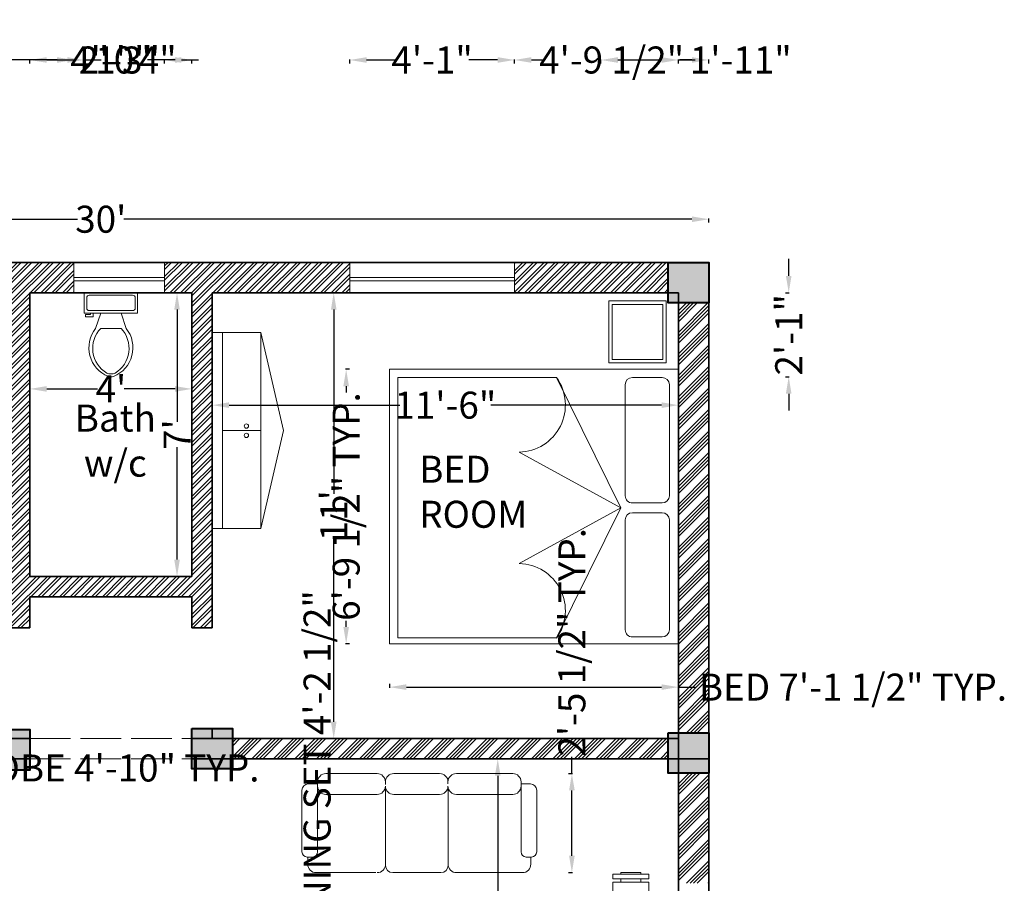
# Model space of a CAD drawing. Units: inches. Extents: x -52 to 493, y -432 to 100.
# Tile 5 of 5: x 163 to 454, y -155 to 100. Entities that reach past the tile are written whole.
import ezdxf

# ---------------------------------------------------------------- set-up
doc = ezdxf.new("R2010")
doc.units = ezdxf.units.IN
doc.header["$MEASUREMENT"] = 0
doc.linetypes.add('ACAD_ISO02W100', pattern=[15, 12, -3])
for name, color, linetype, lineweight in [('A-ANNO-DIMS', 2, 'Continuous', 18), ('A-AREA-IDEN', 7, 'Continuous', 25), ('A-COLS', 7, 'Continuous', 40), ('A-FLOR-FIXT', 9, 'Continuous', 18), ('A-FURN', 8, 'Continuous', 18), ('A-GLAZ', 4, 'Continuous', 18), ('A-WALL', 7, 'Continuous', 35), ('A-WALL-OVHD', 7, 'ACAD_ISO02W100', 18), ('A-WALL-PATT', 8, 'Continuous', 13)]:
    doc.layers.add(name, color=color, linetype=linetype, lineweight=lineweight)
doc.styles.get("Standard").update_dxf_attribs({"font": 'arial.ttf'})
doc.dimstyles.get("Standard").update_dxf_attribs({"dimtxt": 8, "dimasz": 5, "dimexe": 0.18, "dimexo": 0.0625, "dimgap": 0.09, "dimtad": 0, "dimdec": 0, "dimzin": 0, "dimdsep": 46, "dimlunit": 3, "dimtxsty": 'Standard', "dimcen": 0.09, "dimadec": 0, "dimazin": 0, "dimtfac": 1, "dimtdec": 0, "dimtofl": 0, "dimtmove": 0, "dimatfit": 3, "dimfxl": 1, "dimfxlon": 1, "dimtolj": 1, "dimtzin": 0, "dimarcsym": 0})

# ---------------------------------------------------------------- blocks, each defined once
blk = doc.blocks.new('*U4')
for p, q in [((9.5, -6), (9.5, -2)), ((-10, -8.5), (-8, -8.5)), ((-10, -9.5), (-10, -8.5)), ((-7, -9.5), (-10, -9.5)), ((-8, -8.5), (-8, -8)), ((-7, -8), (-7, -9.5)), ((-4, -8), (-6, -14)), ((4, -8), (6, -14)), ((4, -14), (-4, -14))]:
    blk.add_line(p, q)
blk.add_lwpolyline([(10.5, -8), (10.5, 0), (-10.5, 0), (-10.5, -8)], close=True)
for points in [[(-9.5, -2), (-9.5, -6)], [(8.5, -1), (-8.5, -1)], [(-8.5, -7), (8.5, -7)]]:
    blk.add_lwpolyline(points)
for centre, radius, start, end in [((-8.62, -1.88), 0.884, 81.8699, 188.1301), ((8.62, -1.88), 0.884, 351.8699, 98.1301), ((-8.62, -6.12), 0.884, 171.8699, 278.1301), ((8.62, -6.12), 0.884, 261.8699, 8.1301), ((3.52, -21.58), 12.17, 141.4691, 247.9714), ((4.2, -21.82), 11.33, 136.3677, 238.9468), ((-3.52, -21.58), 12.17, 292.0284, 38.5307), ((-4.2, -21.82), 11.33, 301.053, 43.6321), ((0, -27.88), 4, 245.7318, 294.2682), ((0, -29), 4, 254.8605, 285.1395)]:
    blk.add_arc(centre, radius, start, end)
blk = doc.blocks.new('A$C46517758')
for p, q in [((0, 0), (0, 2)), ((0, 2), (1.9, 2)), ((1.9, 2), (1.9, 0)), ((0.8752, 1.9376), (0.1067, 1.9376)), ((1.8026, 1.9376), (1.0424, 1.9376)), ((0.0567, 1.8876), (0.0567, 1.6816)), ((0.9252, 1.6816), (0.9252, 1.8876)), ((0.9924, 1.6816), (0.9924, 1.8876)), ((1.8526, 1.6816), (1.8526, 1.8876)), ((0.9588, 1.6019), (0.0567, 1.1563)), ((0.1067, 1.6316), (0.8752, 1.6316)), ((0.5728, 0.8979), (0.9588, 1.6019)), ((1.8589, 1.1563), (0.9588, 1.6019)), ((1.3448, 0.8979), (0.9588, 1.6019)), ((1.0424, 1.6316), (1.8026, 1.6316)), ((0.0567, 1.1563), (0.0567, 0.0572)), ((1.8589, 0.0572), (1.8589, 1.1563)), ((0.0567, 0.0572), (1.8589, 0.0572)), ((1.9, 0), (0, 0))]:
    blk.add_line(p, q)
for centre, radius, start, end in [((0.1067, 1.8876), 0.05, 90, 180), ((0.8752, 1.8876), 0.05, 0, 90), ((1.0424, 1.8876), 0.05, 90, 180), ((1.8026, 1.8876), 0.05, 0, 90), ((0.1067, 1.6816), 0.05, 180, 270), ((0.8752, 1.6816), 0.05, 270, 0), ((1.0424, 1.6816), 0.05, 180, 270), ((1.8026, 1.6816), 0.05, 270, 0), ((0.2469, 0.8917), 0.3259, 1.08529, 125.71503), ((1.6707, 0.8917), 0.3259, 54.28497, 178.91471)]:
    blk.add_arc(centre, radius, start, end)
blk = doc.blocks.new('A$C0876780F')
for p, q in [((0.72, 0.95), (0.23, 0.95)), ((1.32, 0.95), (0.88, 0.95)), ((1.48, 0.95), (2.02, 0.95)), ((0.15, 0.85), (0.06, 0.85)), ((0.15, 0.87), (0.15, 0.8444)), ((0.15, 0.87), (0.15, 0.85)), ((0.15, 0.21), (0.15, 0.85)), ((0.8, 0.85), (0.8, 0.87)), ((0.8, 0.87), (0.8, 0.85)), ((0.8, 0.87), (0.8, 0.8444)), ((1.4, 0.85), (1.4, 0.87)), ((1.4, 0.85), (1.4, 0.87)), ((2.1, 0.87), (2.1, 0.85)), ((2.1, 0.87), (2.1, 0.8444)), ((2.1, 0.21), (2.1, 0.85)), ((2.1, 0.85), (2.19, 0.85)), ((0, 0.79), (0, 0.21)), ((0.8011, 0.8204), (0.8011, 0.08)), ((1.4014, 0.08), (1.4014, 0.803)), ((2.25, 0.79), (2.25, 0.21)), ((0.72, 0.75), (0.23, 0.75)), ((1.32, 0.75), (0.88, 0.75)), ((1.48, 0.75), (2.02, 0.75)), ((0, 0.21), (0, 0.2)), ((0.15, 0.2), (0.15, 0.25)), ((2.1, 0.2), (2.1, 0.25)), ((2.25, 0.21), (2.25, 0.2)), ((0.05, 0.15), (0.1, 0.15)), ((0.056, 0.15), (0.056, 0.08)), ((2.2, 0.15), (2.15, 0.15)), ((2.194, 0.15), (2.194, 0.08)), ((0.136, 0), (0.7093, 0)), ((0.8011, 0.07), (0.8011, 0.08)), ((0.8711, 0), (1.3314, 0)), ((1.4014, 0.07), (1.4014, 0.08)), ((2.114, 0), (1.48, 0))]:
    blk.add_line(p, q)
for centre, radius, start, end in [((0.23, 0.87), 0.08, 90, 180), ((0.72, 0.87), 0.08, 0, 90), ((0.88, 0.87), 0.08, 90, 180), ((1.32, 0.87), 0.08, 0, 90), ((1.48, 0.87), 0.08, 90, 180), ((2.02, 0.87), 0.08, 0, 90), ((0.06, 0.79), 0.06, 90, 180), ((2.19, 0.79), 0.06, 0, 90), ((0.23, 0.83), 0.08, 180, 270), ((0.23, 0.83), 0.08, 180, 270), ((0.72, 0.83), 0.08, 270, 0), ((0.88, 0.83), 0.08, 180, 270), ((0.88, 0.83), 0.08, 180, 270), ((1.32, 0.83), 0.08, 270, 0), ((1.48, 0.83), 0.08, 180, 270), ((2.02, 0.83), 0.08, 270, 0), ((2.02, 0.83), 0.08, 270, 0), ((0.05, 0.2), 0.05, 180, 270), ((0.1, 0.2), 0.05, 270, 0), ((0.09, 0.21), 0.06, 350.53768, 0), ((2.16, 0.21), 0.06, 180, 189.46232), ((2.15, 0.2), 0.05, 180, 270), ((2.2, 0.2), 0.05, 270, 0), ((0.136, 0.08), 0.08, 180, 270), ((0.7211, 0.08), 0.08, 270, 0), ((0.8711, 0.07), 0.07, 180, 270), ((1.3314, 0.07), 0.07, 270, 0), ((1.4814, 0.08), 0.08, 180, 270), ((2.114, 0.08), 0.08, 270, 0)]:
    blk.add_arc(centre, radius, start, end)
blk = doc.blocks.new('*D13')
at = {"layer": 'A-ANNO-DIMS', "color": 0, "lineweight": -2, "transparency": 16777216}
for p, q in [((165.65, -9.09), (165.65, -8.91)), ((170.65, -9.09), (185.72, -9.09)), ((208.65, -9.09), (193.58, -9.09)), ((213.65, -9.09), (213.65, -8.91))]:
    blk.add_line(p, q, dxfattribs=at)
at = {"layer": 'A-ANNO-DIMS', "color": 0, "transparency": 16777216}
for points in [[(170.65, -8.26), (170.65, -9.93), (165.65, -9.09)], [(208.65, -8.26), (208.65, -9.93), (213.65, -9.09)]]:
    blk.add_solid(points, dxfattribs=at)
at = {"layer": 'Defpoints', "color": 0, "transparency": 16777216}
for p in [(165.65, -9.09), (213.65, -9.09), (213.65, -9.09)]:
    blk.add_point(p, dxfattribs=at)
at = {"layer": 'A-ANNO-DIMS', "color": 0, "transparency": 16777216, "insert": (189.65, -9.09), "char_height": 8, "attachment_point": 5}
blk.add_mtext("\\A1;4'", dxfattribs=at)
blk = doc.blocks.new('*D14')
at = {"layer": 'A-ANNO-DIMS', "color": 0, "lineweight": -2, "transparency": 16777216}
for p, q in [((208.22, 19.38), (209.4, 19.38)), ((209.22, 14.38), (209.22, -18.88)), ((209.22, -59.62), (209.22, -26.35)), ((208.55, -64.62), (209.4, -64.62))]:
    blk.add_line(p, q, dxfattribs=at)
at = {"layer": 'A-ANNO-DIMS', "color": 0, "transparency": 16777216}
for points in [[(208.39, 14.38), (210.05, 14.38), (209.22, 19.38)], [(208.39, -59.62), (210.05, -59.62), (209.22, -64.62)]]:
    blk.add_solid(points, dxfattribs=at)
at = {"layer": 'Defpoints', "color": 0, "transparency": 16777216}
for p in [(205.54, 19.38), (209.22, 19.38), (208.49, -64.62)]:
    blk.add_point(p, dxfattribs=at)
at = {"layer": 'A-ANNO-DIMS', "color": 0, "transparency": 16777216, "insert": (209.22, -22.62), "char_height": 8, "attachment_point": 5, "rotation": 90}
blk.add_mtext("\\A1;7'", dxfattribs=at)
blk = doc.blocks.new('*D15')
at = {"layer": 'A-ANNO-DIMS', "color": 0, "lineweight": -2, "transparency": 16777216}
for p, q in [((219.65, -12.9), (219.65, -14.08)), ((224.65, -13.9), (275.19, -13.9)), ((352.65, -13.9), (302.1, -13.9)), ((357.65, -12.9), (357.65, -14.08))]:
    blk.add_line(p, q, dxfattribs=at)
at = {"layer": 'A-ANNO-DIMS', "color": 0, "transparency": 16777216}
for points in [[(224.65, -13.06), (224.65, -14.73), (219.65, -13.9)], [(352.65, -13.06), (352.65, -14.73), (357.65, -13.9)]]:
    blk.add_solid(points, dxfattribs=at)
at = {"layer": 'Defpoints', "color": 0, "transparency": 16777216}
for p in [(219.65, -3.74), (357.65, -3.74), (357.65, -13.9)]:
    blk.add_point(p, dxfattribs=at)
at = {"layer": 'A-ANNO-DIMS', "color": 0, "transparency": 16777216, "insert": (288.65, -13.9), "char_height": 8, "attachment_point": 5}
blk.add_mtext('\\A1;11\'-6"', dxfattribs=at)
blk = doc.blocks.new('*D16')
at = {"layer": 'A-ANNO-DIMS', "color": 0, "lineweight": -2, "transparency": 16777216}
for p, q in [((255.93, 19.38), (255.43, 19.38)), ((255.61, 14.38), (255.61, -40.11)), ((255.61, -107.62), (255.61, -53.12)), ((255.93, -112.62), (255.43, -112.62))]:
    blk.add_line(p, q, dxfattribs=at)
at = {"layer": 'A-ANNO-DIMS', "color": 0, "transparency": 16777216}
for points in [[(254.78, 14.38), (256.44, 14.38), (255.61, 19.38)], [(254.78, -107.62), (256.44, -107.62), (255.61, -112.62)]]:
    blk.add_solid(points, dxfattribs=at)
at = {"layer": 'Defpoints', "color": 0, "transparency": 16777216}
for p in [(255.61, 19.38), (256, 19.38), (256, -112.62)]:
    blk.add_point(p, dxfattribs=at)
at = {"layer": 'A-ANNO-DIMS', "color": 0, "transparency": 16777216, "insert": (255.61, -46.62), "char_height": 8, "attachment_point": 5, "rotation": 90}
blk.add_mtext("\\A1;11'", dxfattribs=at)
blk = doc.blocks.new('*D22')
at = {"layer": 'A-ANNO-DIMS', "color": 0, "lineweight": -2, "transparency": 16777216}
for p, q in [((6.65, 40.15), (6.65, 41.33)), ((11.65, 41.15), (179.77, 41.15)), ((361.65, 41.15), (193.52, 41.15)), ((366.65, 40.15), (366.65, 41.33))]:
    blk.add_line(p, q, dxfattribs=at)
at = {"layer": 'A-ANNO-DIMS', "color": 0, "transparency": 16777216}
for points in [[(11.65, 41.98), (11.65, 40.31), (6.65, 41.15)], [(361.65, 41.98), (361.65, 40.31), (366.65, 41.15)]]:
    blk.add_solid(points, dxfattribs=at)
at = {"layer": 'Defpoints', "color": 0, "transparency": 16777216}
for p in [(366.65, 41.15), (6.65, 28.38), (366.65, 28.38)]:
    blk.add_point(p, dxfattribs=at)
at = {"layer": 'A-ANNO-DIMS', "color": 0, "transparency": 16777216, "insert": (186.65, 41.15), "char_height": 8, "attachment_point": 5}
blk.add_mtext("\\A1;30'", dxfattribs=at)
blk = doc.blocks.new('*D26')
at = {"layer": 'A-ANNO-DIMS', "color": 0, "lineweight": -2, "transparency": 16777216}
for p, q in [((305.16, -118.62), (303.98, -118.62)), ((304.16, -123.62), (304.16, -178.11)), ((304.16, -245.62), (304.16, -191.12)), ((305.16, -250.62), (303.98, -250.62))]:
    blk.add_line(p, q, dxfattribs=at)
at = {"layer": 'A-ANNO-DIMS', "color": 0, "transparency": 16777216}
for points in [[(303.33, -123.62), (305, -123.62), (304.16, -118.62)], [(303.33, -245.62), (305, -245.62), (304.16, -250.62)]]:
    blk.add_solid(points, dxfattribs=at)
at = {"layer": 'Defpoints', "color": 0, "transparency": 16777216}
for p in [(304.16, -118.62), (307.2, -118.62), (312.14, -250.62)]:
    blk.add_point(p, dxfattribs=at)
at = {"layer": 'A-ANNO-DIMS', "color": 0, "transparency": 16777216, "insert": (304.16, -184.62), "char_height": 8, "attachment_point": 5, "rotation": 90}
blk.add_mtext("\\A1;11'", dxfattribs=at)
blk = doc.blocks.new('COL-12X12')
h = blk.add_hatch(color=256)
h.dxf.hatch_style = 1
h.paths.add_polyline_path([(12, 12), (0, 12), (0, 0), (12, 0)])
blk.add_lwpolyline([(0, 12), (12, 12), (12, 0), (0, 0)], close=True)
blk = doc.blocks.new('WARDROBE-DOUBLE')
for p, q in [((0, 14.42), (29.03, 21.14)), ((29.03, 21.14), (58.05, 14.42)), ((0, 3.04), (0, 14.42)), ((0, 14.42), (58.05, 14.42)), ((29.03, 14.42), (29.03, 3.04)), ((58.05, 14.42), (58.05, 3.04)), ((0, 0), (0, 3.04)), ((0, 3.04), (58.05, 3.04)), ((58.05, 3.04), (58.05, 0))]:
    blk.add_line(p, q)
for centre in [(27.68, 10.11), (30.45, 10.11)]:
    blk.add_circle(centre, 0.653)
blk = doc.blocks.new('CHAIR-DINING')
for p, q in [((10.59, 12.94), (0, 12.94)), ((0, 12.94), (0, 11.53)), ((8.23, 13.41), (2.35, 13.41)), ((2.35, 13.41), (2.35, 12.94)), ((8.23, 12.94), (8.23, 13.41)), ((10.59, 11.53), (10.59, 12.94)), ((10.59, 11.53), (0, 11.53)), ((10.59, 10.59), (0, 10.59)), ((0, 10.59), (0, 0)), ((2.35, 11.53), (2.35, 10.59)), ((8.23, 10.59), (8.23, 11.53)), ((10.59, 0), (10.59, 10.59)), ((0, 0), (10.59, 0))]:
    blk.add_line(p, q)
blk = doc.blocks.new('*D38')
at = {"layer": 'A-ANNO-DIMS', "color": 0, "lineweight": -2, "transparency": 16777216}
for p, q in [((50.07, -120.32), (50.07, -121.5)), ((55.07, -121.32), (103.12, -121.32)), ((108.12, -120.32), (108.12, -121.5)), ((108.12, -121.32), (113.12, -121.32))]:
    blk.add_line(p, q, dxfattribs=at)
at = {"layer": 'A-ANNO-DIMS', "color": 0, "transparency": 16777216}
for points in [[(55.07, -120.49), (55.07, -122.16), (50.07, -121.32)], [(103.12, -120.49), (103.12, -122.16), (108.12, -121.32)]]:
    blk.add_solid(points, dxfattribs=at)
at = {"layer": 'Defpoints', "color": 0, "transparency": 16777216}
for p in [(50.07, -112.62), (108.12, -112.62), (108.12, -121.32)]:
    blk.add_point(p, dxfattribs=at)
at = {"layer": 'A-ANNO-DIMS', "color": 0, "transparency": 16777216, "insert": (175.33, -121.32), "char_height": 8, "attachment_point": 5}
blk.add_mtext('\\A1;WARDROBE 4\'-10" TYP.', dxfattribs=at)
blk = doc.blocks.new('*D42')
at = {"layer": 'A-ANNO-DIMS', "color": 0, "lineweight": -2, "transparency": 16777216}
for p, q in [((272.12, -96.38), (272.12, -97.56)), ((277.12, -97.38), (352.65, -97.38)), ((357.65, -96.38), (357.65, -97.56)), ((357.65, -97.38), (362.65, -97.38))]:
    blk.add_line(p, q, dxfattribs=at)
at = {"layer": 'A-ANNO-DIMS', "color": 0, "transparency": 16777216}
for points in [[(277.12, -96.54), (277.12, -98.21), (272.12, -97.38)], [(352.65, -96.54), (352.65, -98.21), (357.65, -97.38)]]:
    blk.add_solid(points, dxfattribs=at)
at = {"layer": 'Defpoints', "color": 0, "transparency": 16777216}
for p in [(272.12, -84.55), (357.65, -84.55), (357.65, -97.38)]:
    blk.add_point(p, dxfattribs=at)
at = {"layer": 'A-ANNO-DIMS', "color": 0, "transparency": 16777216, "insert": (409.31, -97.38), "char_height": 8, "attachment_point": 5}
blk.add_mtext('\\A1;BED 7\'-1 1/2" TYP.', dxfattribs=at)
blk = doc.blocks.new('*D43')
at = {"layer": 'A-ANNO-DIMS', "color": 0, "lineweight": -2, "transparency": 16777216}
for p, q in [((260.29, -3.29), (259.11, -3.29)), ((259.29, -8.29), (259.29, -10.11)), ((259.29, -79.55), (259.29, -77.74)), ((260.29, -84.55), (259.11, -84.55))]:
    blk.add_line(p, q, dxfattribs=at)
at = {"layer": 'A-ANNO-DIMS', "color": 0, "transparency": 16777216}
for points in [[(258.46, -8.29), (260.12, -8.29), (259.29, -3.29)], [(258.46, -79.55), (260.12, -79.55), (259.29, -84.55)]]:
    blk.add_solid(points, dxfattribs=at)
at = {"layer": 'Defpoints', "color": 0, "transparency": 16777216}
for p in [(272.12, -3.29), (259.29, -84.55), (272.12, -84.55)]:
    blk.add_point(p, dxfattribs=at)
at = {"layer": 'A-ANNO-DIMS', "color": 0, "transparency": 16777216, "insert": (259.29, -43.92), "char_height": 8, "attachment_point": 5, "rotation": 90}
blk.add_mtext('\\A1;6\'-9 1/2" TYP.', dxfattribs=at)
blk = doc.blocks.new('*D46')
at = {"layer": 'A-ANNO-DIMS', "color": 0, "lineweight": -2, "transparency": 16777216}
for p, q in [((246.2, -161.73), (246.2, -162.91)), ((251.2, -162.73), (310.69, -162.73)), ((315.69, -161.73), (315.69, -162.91)), ((315.69, -162.73), (320.69, -162.73))]:
    blk.add_line(p, q, dxfattribs=at)
at = {"layer": 'A-ANNO-DIMS', "color": 0, "transparency": 16777216}
for points in [[(251.2, -161.9), (251.2, -163.56), (246.2, -162.73)], [(310.69, -161.9), (310.69, -163.56), (315.69, -162.73)]]:
    blk.add_solid(points, dxfattribs=at)
at = {"layer": 'Defpoints', "color": 0, "transparency": 16777216}
for p in [(246.2, -152.31), (315.69, -152.31), (315.69, -162.73)]:
    blk.add_point(p, dxfattribs=at)
at = {"layer": 'A-ANNO-DIMS', "color": 0, "transparency": 16777216, "insert": (371.23, -162.73), "char_height": 8, "attachment_point": 5}
blk.add_mtext('\\A1;SOFA 5\'-9 1/2" TYP.', dxfattribs=at)
blk = doc.blocks.new('*D47')
at = {"layer": 'A-ANNO-DIMS', "color": 0, "lineweight": -2, "transparency": 16777216}
for p, q in [((326.11, -122.97), (326.11, -117.97)), ((325.11, -122.97), (326.29, -122.97)), ((326.11, -147.31), (326.11, -127.97)), ((325.11, -152.31), (326.29, -152.31))]:
    blk.add_line(p, q, dxfattribs=at)
at = {"layer": 'A-ANNO-DIMS', "color": 0, "transparency": 16777216}
for points in [[(325.28, -127.97), (326.95, -127.97), (326.11, -122.97)], [(325.28, -147.31), (326.95, -147.31), (326.11, -152.31)]]:
    blk.add_solid(points, dxfattribs=at)
at = {"layer": 'Defpoints', "color": 0, "transparency": 16777216}
for p in [(315.69, -122.97), (326.11, -122.97), (315.69, -152.31)]:
    blk.add_point(p, dxfattribs=at)
at = {"layer": 'A-ANNO-DIMS', "color": 0, "transparency": 16777216, "insert": (326.11, -84.11), "char_height": 8, "attachment_point": 5, "rotation": 90}
blk.add_mtext('\\A1;2\'-5 1/2" TYP.', dxfattribs=at)
blk = doc.blocks.new('*D48')
at = {"layer": 'A-ANNO-DIMS', "color": 0, "lineweight": -2, "transparency": 16777216}
for p, q in [((250.69, -179.3), (250.69, -174.3)), ((251.69, -179.3), (250.51, -179.3)), ((250.69, -224.88), (250.69, -184.3)), ((251.69, -229.88), (250.51, -229.88))]:
    blk.add_line(p, q, dxfattribs=at)
at = {"layer": 'A-ANNO-DIMS', "color": 0, "transparency": 16777216}
for points in [[(249.85, -184.3), (251.52, -184.3), (250.69, -179.3)], [(249.85, -224.88), (251.52, -224.88), (250.69, -229.88)]]:
    blk.add_solid(points, dxfattribs=at)
at = {"layer": 'Defpoints', "color": 0, "transparency": 16777216}
for p in [(250.69, -179.3), (258.27, -179.3), (258.27, -229.88)]:
    blk.add_point(p, dxfattribs=at)
at = {"layer": 'A-ANNO-DIMS', "color": 0, "transparency": 16777216, "insert": (250.69, -120.92), "char_height": 8, "attachment_point": 5, "rotation": 90}
blk.add_mtext('\\A1;DINING SET 4\'-2 1/2"', dxfattribs=at)
blk = doc.blocks.new('*D56')
at = {"layer": 'A-ANNO-DIMS', "color": 0, "lineweight": -2, "transparency": 16777216}
for p, q in [((6.65, 87.29), (6.65, 88.47)), ((11.65, 88.29), (79.23, 88.29)), ((173.72, 88.29), (106.14, 88.29)), ((178.72, 87.29), (178.72, 88.47))]:
    blk.add_line(p, q, dxfattribs=at)
at = {"layer": 'A-ANNO-DIMS', "color": 0, "transparency": 16777216}
for points in [[(11.65, 89.13), (11.65, 87.46), (6.65, 88.29)], [(173.72, 89.13), (173.72, 87.46), (178.72, 88.29)]]:
    blk.add_solid(points, dxfattribs=at)
at = {"layer": 'Defpoints', "color": 0, "transparency": 16777216}
for p in [(178.72, 88.29), (6.65, 28.38), (178.72, 28.38)]:
    blk.add_point(p, dxfattribs=at)
at = {"layer": 'A-ANNO-DIMS', "color": 0, "transparency": 16777216, "insert": (92.68, 88.29), "char_height": 8, "attachment_point": 5}
blk.add_mtext('\\A1;14\'-4"', dxfattribs=at)
blk = doc.blocks.new('*D57')
at = {"layer": 'A-ANNO-DIMS', "color": 0, "lineweight": -2, "transparency": 16777216}
for p, q in [((173.72, 88.29), (168.72, 88.29)), ((178.72, 87.29), (178.72, 88.47)), ((205.54, 87.29), (205.54, 88.47)), ((210.54, 88.29), (215.54, 88.29))]:
    blk.add_line(p, q, dxfattribs=at)
at = {"layer": 'A-ANNO-DIMS', "color": 0, "transparency": 16777216}
for points in [[(173.72, 89.13), (173.72, 87.46), (178.72, 88.29)], [(210.54, 89.13), (210.54, 87.46), (205.54, 88.29)]]:
    blk.add_solid(points, dxfattribs=at)
at = {"layer": 'Defpoints', "color": 0, "transparency": 16777216}
for p in [(205.54, 88.29), (178.72, 28.38), (205.54, 28.38)]:
    blk.add_point(p, dxfattribs=at)
at = {"layer": 'A-ANNO-DIMS', "color": 0, "transparency": 16777216, "insert": (192.13, 88.29), "char_height": 8, "attachment_point": 5}
blk.add_mtext('\\A1;2\'-3"', dxfattribs=at)
blk = doc.blocks.new('*D58')
at = {"layer": 'A-ANNO-DIMS', "color": 0, "lineweight": -2, "transparency": 16777216}
for p, q in [((260.34, 87.29), (260.34, 88.47)), ((265.34, 88.29), (273.84, 88.29)), ((304.11, 88.29), (295.61, 88.29)), ((309.11, 87.29), (309.11, 88.47))]:
    blk.add_line(p, q, dxfattribs=at)
at = {"layer": 'A-ANNO-DIMS', "color": 0, "transparency": 16777216}
for points in [[(265.34, 89.13), (265.34, 87.46), (260.34, 88.29)], [(304.11, 89.13), (304.11, 87.46), (309.11, 88.29)]]:
    blk.add_solid(points, dxfattribs=at)
at = {"layer": 'Defpoints', "color": 0, "transparency": 16777216}
for p in [(309.11, 88.29), (260.34, 28.38), (309.11, 28.38)]:
    blk.add_point(p, dxfattribs=at)
at = {"layer": 'A-ANNO-DIMS', "color": 0, "transparency": 16777216, "insert": (284.73, 88.29), "char_height": 8, "attachment_point": 5}
blk.add_mtext('\\A1;4\'-1"', dxfattribs=at)
blk = doc.blocks.new('*D59')
at = {"layer": 'A-ANNO-DIMS', "color": 0, "lineweight": -2, "transparency": 16777216}
for p, q in [((309.11, 87.29), (309.11, 88.47)), ((314.11, 88.29), (317.67, 88.29)), ((361.65, 88.29), (358.08, 88.29)), ((366.65, 87.29), (366.65, 88.47))]:
    blk.add_line(p, q, dxfattribs=at)
at = {"layer": 'A-ANNO-DIMS', "color": 0, "transparency": 16777216}
for points in [[(314.11, 89.13), (314.11, 87.46), (309.11, 88.29)], [(361.65, 89.13), (361.65, 87.46), (366.65, 88.29)]]:
    blk.add_solid(points, dxfattribs=at)
at = {"layer": 'Defpoints', "color": 0, "transparency": 16777216}
for p in [(366.65, 88.29), (309.11, 28.38), (366.65, 28.38)]:
    blk.add_point(p, dxfattribs=at)
at = {"layer": 'A-ANNO-DIMS', "color": 0, "transparency": 16777216, "insert": (337.88, 88.29), "char_height": 8, "attachment_point": 5}
blk.add_mtext('\\A1;4\'-9 1/2"', dxfattribs=at)
blk = doc.blocks.new('*D70')
at = {"layer": 'A-ANNO-DIMS', "color": 0, "lineweight": -2, "transparency": 16777216}
for p, q in [((165.65, 87.29), (165.65, 88.47)), ((170.65, 88.29), (178.76, 88.29)), ((208.65, 88.29), (200.53, 88.29)), ((213.65, 87.29), (213.65, 88.47))]:
    blk.add_line(p, q, dxfattribs=at)
at = {"layer": 'A-ANNO-DIMS', "color": 0, "transparency": 16777216}
for points in [[(170.65, 89.13), (170.65, 87.46), (165.65, 88.29)], [(208.65, 89.13), (208.65, 87.46), (213.65, 88.29)]]:
    blk.add_solid(points, dxfattribs=at)
at = {"layer": 'Defpoints', "color": 0, "transparency": 16777216}
for p in [(213.65, 88.29), (165.65, -112.62), (213.65, -112.62)]:
    blk.add_point(p, dxfattribs=at)
at = {"layer": 'A-ANNO-DIMS', "color": 0, "transparency": 16777216, "insert": (189.65, 88.29), "char_height": 8, "attachment_point": 5}
blk.add_mtext('\\A1;4\'-0"', dxfattribs=at)
blk = doc.blocks.new('*D71')
at = {"layer": 'A-ANNO-DIMS', "color": 0, "lineweight": -2, "transparency": 16777216}
for p, q in [((-17, -65.62), (-17, -60.62)), ((-16, -70.62), (-17.18, -70.62)), ((-16, -79.87), (-17.18, -79.87)), ((-17, -84.87), (-17, -89.87))]:
    blk.add_line(p, q, dxfattribs=at)
at = {"layer": 'A-ANNO-DIMS', "color": 0, "transparency": 16777216}
for points in [[(-17.84, -65.62), (-16.17, -65.62), (-17, -70.62)], [(-17.84, -84.87), (-16.17, -84.87), (-17, -79.87)]]:
    blk.add_solid(points, dxfattribs=at)
at = {"layer": 'Defpoints', "color": 0, "transparency": 16777216}
for p in [(165.65, -70.62), (-17, -79.87), (165.65, -79.87)]:
    blk.add_point(p, dxfattribs=at)
at = {"layer": 'A-ANNO-DIMS', "color": 0, "transparency": 16777216, "insert": (-17, -109.92), "char_height": 8, "attachment_point": 5, "rotation": 90}
blk.add_mtext('\\A1;0\'-9 1/2"', dxfattribs=at)
blk = doc.blocks.new('*D74')
at = {"layer": 'A-ANNO-DIMS', "color": 0, "lineweight": -2, "transparency": 16777216}
for p, q in [((334.72, 87.29), (334.72, 88.47)), ((339.72, 88.29), (352.65, 88.29)), ((357.65, 87.29), (357.65, 88.47)), ((357.65, 88.29), (362.65, 88.29))]:
    blk.add_line(p, q, dxfattribs=at)
at = {"layer": 'A-ANNO-DIMS', "color": 0, "transparency": 16777216}
for points in [[(339.72, 89.13), (339.72, 87.46), (334.72, 88.29)], [(352.65, 89.13), (352.65, 87.46), (357.65, 88.29)]]:
    blk.add_solid(points, dxfattribs=at)
at = {"layer": 'Defpoints', "color": 0, "transparency": 16777216}
for p in [(357.65, 88.29), (334.72, -335.93), (357.65, -358.62)]:
    blk.add_point(p, dxfattribs=at)
at = {"layer": 'A-ANNO-DIMS', "color": 0, "transparency": 16777216, "insert": (376.1, 88.29), "char_height": 8, "attachment_point": 5}
blk.add_mtext('\\A1;1\'-11"', dxfattribs=at)
blk = doc.blocks.new('*D78')
at = {"layer": 'A-ANNO-DIMS', "color": 0, "lineweight": -2, "transparency": 16777216}
for p, q in [((390.3, 24.38), (390.3, 29.38)), ((389.3, 19.38), (390.48, 19.38)), ((389.3, -5.51), (390.48, -5.51)), ((390.3, -10.51), (390.3, -15.51))]:
    blk.add_line(p, q, dxfattribs=at)
at = {"layer": 'A-ANNO-DIMS', "color": 0, "transparency": 16777216}
for points in [[(389.46, 24.38), (391.13, 24.38), (390.3, 19.38)], [(389.46, -10.51), (391.13, -10.51), (390.3, -5.51)]]:
    blk.add_solid(points, dxfattribs=at)
at = {"layer": 'Defpoints', "color": 0, "transparency": 16777216}
for p in [(197.57, 19.38), (189.65, -5.51), (390.3, -5.51)]:
    blk.add_point(p, dxfattribs=at)
at = {"layer": 'A-ANNO-DIMS', "color": 0, "transparency": 16777216, "insert": (390.3, 6.94), "char_height": 8, "attachment_point": 5, "rotation": 90}
blk.add_mtext('\\A1;2\'-1"', dxfattribs=at)
blk = doc.blocks.new('*D79')
at = {"layer": 'A-ANNO-DIMS', "color": 0, "lineweight": -2, "transparency": 16777216}
for p, q in [((181.73, -419.22), (181.73, -420.4)), ((197.57, -419.22), (197.57, -420.4)), ((186.73, -420.22), (192.57, -420.22)), ((197.57, -420.22), (202.57, -420.22))]:
    blk.add_line(p, q, dxfattribs=at)
at = {"layer": 'A-ANNO-DIMS', "color": 0, "transparency": 16777216}
for points in [[(186.73, -419.39), (186.73, -421.06), (181.73, -420.22)], [(192.57, -419.39), (192.57, -421.06), (197.57, -420.22)]]:
    blk.add_solid(points, dxfattribs=at)
at = {"layer": 'Defpoints', "color": 0, "transparency": 16777216}
for p in [(181.73, 19.38), (197.57, 19.38), (197.57, -420.22)]:
    blk.add_point(p, dxfattribs=at)
at = {"layer": 'A-ANNO-DIMS', "color": 0, "transparency": 16777216, "insert": (212.91, -420.22), "char_height": 8, "attachment_point": 5}
blk.add_mtext('\\A1;1\'-4"', dxfattribs=at)
blk = doc.blocks.new('*D80')
at = {"layer": 'A-ANNO-DIMS', "color": 0, "lineweight": -2, "transparency": 16777216}
for p, q in [((165.65, 87.29), (165.65, 88.47)), ((170.65, 88.29), (176.73, 88.29)), ((181.73, 87.29), (181.73, 88.47)), ((181.73, 88.29), (186.73, 88.29))]:
    blk.add_line(p, q, dxfattribs=at)
at = {"layer": 'A-ANNO-DIMS', "color": 0, "transparency": 16777216}
for points in [[(170.65, 89.13), (170.65, 87.46), (165.65, 88.29)], [(176.73, 89.13), (176.73, 87.46), (181.73, 88.29)]]:
    blk.add_solid(points, dxfattribs=at)
at = {"layer": 'Defpoints', "color": 0, "transparency": 16777216}
for p in [(181.73, 88.29), (165.65, 19.38), (181.73, 19.38)]:
    blk.add_point(p, dxfattribs=at)
at = {"layer": 'A-ANNO-DIMS', "color": 0, "transparency": 16777216, "insert": (197.07, 88.29), "char_height": 8, "attachment_point": 5}
blk.add_mtext('\\A1;1\'-4"', dxfattribs=at)
blk = doc.blocks.new('*D81')
at = {"layer": 'A-ANNO-DIMS', "color": 0, "lineweight": -2, "transparency": 16777216}
for p, q in [((159.65, -419.22), (159.65, -420.4)), ((165.65, -419.22), (165.65, -420.4)), ((154.65, -420.22), (149.65, -420.22)), ((170.65, -420.22), (175.65, -420.22))]:
    blk.add_line(p, q, dxfattribs=at)
at = {"layer": 'A-ANNO-DIMS', "color": 0, "transparency": 16777216}
for points in [[(154.65, -419.39), (154.65, -421.06), (159.65, -420.22)], [(170.65, -419.39), (170.65, -421.06), (165.65, -420.22)]]:
    blk.add_solid(points, dxfattribs=at)
at = {"layer": 'Defpoints', "color": 0, "transparency": 16777216}
for p in [(159.65, -79.87), (165.65, -79.87), (165.65, -420.22)]:
    blk.add_point(p, dxfattribs=at)
at = {"layer": 'A-ANNO-DIMS', "color": 0, "transparency": 16777216, "insert": (186.37, -420.22), "char_height": 8, "attachment_point": 5}
blk.add_mtext('\\A1;0\'-6"', dxfattribs=at)

msp = doc.modelspace()

# ---------------------------------------------------------------- hatches: boundary and pattern name
at = {"layer": 'A-WALL-PATT'}
h = msp.add_hatch(dxfattribs=at)
h.set_pattern_fill('ANSI32', color=256, scale=6)
h.paths.add_polyline_path([(178.72, 28.38), (18.65, 28.38), (18.65, 19.38), (159.65, 19.38), (159.65, -79.87), (165.65, -79.87), (165.65, -70.62), (213.65, -70.62), (213.65, -79.87), (219.65, -79.87), (219.65, 19.38), (260.34, 19.38), (260.34, 28.38), (205.54, 28.38), (205.54, 19.38), (213.65, 19.38), (213.65, -64.62), (165.65, -64.62), (165.65, 19.38), (178.72, 19.38)])
h.paths.add_polyline_path([(354.65, 28.38), (309.11, 28.38), (309.11, 19.38), (354.65, 19.38)])
h = msp.add_hatch(dxfattribs=at)
h.set_pattern_fill('ANSI34', color=256, scale=6)
h.paths.add_polyline_path([(366.65, 16.38), (357.65, 16.38), (357.65, -110.87), (366.65, -110.87)])
h.paths.add_polyline_path([(15.65, 16.38), (6.65, 16.38), (6.65, -24.71), (15.65, -24.71)])
h.paths.add_polyline_path([(15.65, -82.5), (6.65, -82.5), (6.65, -109.57), (15.65, -109.57)])
h.paths.add_polyline_path([(366.65, -122.87), (357.65, -122.87), (357.65, -155.46), (366.65, -155.46)])
h.paths.add_polyline_path([(354.65, -112.62), (225.65, -112.62), (225.65, -118.62), (354.65, -118.62)])
h.paths.add_polyline_path([(153.65, -112.62), (18.65, -112.62), (18.65, -118.62), (153.65, -118.62)])

# ---------------------------------------------------------------- linework, layer by layer
at = {"layer": 'A-FURN'}
for points in [[(337.07, 16.94), (354.02, 16.94), (354.02, -1.36), (337.07, -1.36)], [(338.07, 15.94), (353.02, 15.94), (353.02, -0.36), (338.07, -0.36)]]:
    msp.add_lwpolyline(points, close=True, dxfattribs=at)
at = {"layer": 'A-GLAZ'}
for p, q in [((178.72, 28.38), (178.72, 19.38)), ((205.54, 28.38), (205.54, 19.38)), ((260.34, 28.38), (260.34, 19.38)), ((309.11, 28.38), (309.11, 19.38)), ((205.54, 23.88), (178.72, 23.88)), ((309.11, 23.88), (260.34, 23.88)), ((205.54, 22.88), (178.72, 22.88)), ((309.11, 22.88), (260.34, 22.88))]:
    msp.add_line(p, q, dxfattribs=at)
at = {"layer": 'A-WALL'}
for p, q in [((6.65, 28.38), (366.65, 28.38)), ((366.65, 28.38), (366.65, -364.62)), ((165.65, 19.38), (165.65, -64.62)), ((165.65, 19.38), (213.65, 19.38)), ((213.65, 19.38), (213.65, -64.62)), ((219.65, 19.38), (219.65, -79.87)), ((219.65, 19.38), (357.65, 19.38)), ((357.65, 19.38), (357.65, -250.62)), ((165.65, -64.62), (213.65, -64.62)), ((165.65, -70.62), (213.65, -70.62)), ((165.65, -70.62), (165.65, -79.87)), ((213.65, -70.62), (213.65, -79.87)), ((165.65, -79.87), (159.65, -79.87)), ((213.65, -79.87), (219.65, -79.87)), ((165.65, -109.95), (165.65, -118.62)), ((213.65, -109.6), (213.65, -118.62)), ((219.65, -109.6), (219.65, -112.62)), ((159.65, -112.62), (165.65, -112.62)), ((213.65, -112.62), (357.65, -112.62)), ((159.65, -118.62), (165.65, -118.62)), ((165.65, -118.62), (165.65, -121.95)), ((213.65, -118.62), (366.65, -118.62))]:
    msp.add_line(p, q, dxfattribs=at)
at = {"layer": 'A-WALL-OVHD'}
for p, q in [((165.65, -112.62), (213.65, -112.62)), ((165.65, -118.62), (213.65, -118.62))]:
    msp.add_line(p, q, dxfattribs=at)

# ---------------------------------------------------------------- block references
at = {"layer": 'A-COLS'}
for p in [(354.65, 16.38), (153.65, -121.95), (213.65, -121.6), (354.65, -122.87)]:
    msp.add_blockref('COL-12X12', p, dxfattribs=at)
at = {"layer": 'A-FLOR-FIXT', "xscale": 0.754322957544484, "yscale": 0.754322957544484, "zscale": 0.754322957544484}
msp.add_blockref('*U4', (189.65, 19.38), dxfattribs=at)
at = {"layer": 'A-FURN', "rotation": 269.9999999999997}
msp.add_blockref('WARDROBE-DOUBLE', (219.65, 7.59), dxfattribs=at)
at = {"layer": 'A-FURN', "xscale": 42.76422276661556, "yscale": 42.76422276661556, "zscale": 42.76422276661556, "rotation": 270}
msp.add_blockref('A$C46517758', (272.12, -3.29), dxfattribs=at)
at = {"layer": 'A-FURN', "xscale": 30.88339250666864, "yscale": 30.88339250666864, "zscale": 30.88339250666864}
msp.add_blockref('A$C0876780F', (246.2, -152.31), dxfattribs=at)
at = {"layer": 'A-FURN'}
msp.add_blockref('CHAIR-DINING', (338.28, -165.71), dxfattribs=at)

# ---------------------------------------------------------------- texts
at = {"layer": 'A-AREA-IDEN', "char_height": 8, "attachment_point": 1}
for s, width, insert in [('\\pxqc;Bath\\Pw/c', 42.7825, (169.57, -13.73)), ('BED\\PROOM', 75.9525, (280.91, -28.87))]:
    msp.add_mtext_dynamic_manual_height_columns(s, width=width, gutter_width=1, heights=[0], dxfattribs=dict(at, insert=insert))

# ---------------------------------------------------------------- dimensions: what is measured, and where the dimension line sits
at = {"layer": 'A-ANNO-DIMS'}
for base, p1, p2, override, picture, middle in [((366.65, 88.29), (309.11, 28.38), (366.65, 28.38), {"dimdec": 1, "dimlfac": 1, "dimrnd": 0, "dimzin": 1, "dimdsep": 46, "dimlunit": 4, "dimfrac": 2}, '*D59', (337.88, 88.29)), ((178.72, 88.29), (6.65, 28.38), (178.72, 28.38), {"dimdec": 1, "dimlfac": 1, "dimrnd": 0, "dimzin": 1, "dimdsep": 46, "dimlunit": 4, "dimfrac": 2}, '*D56', (92.68, 88.29)), ((213.65, 88.29), (165.65, -112.62), (213.65, -112.62), {"dimdec": 1, "dimlfac": 1, "dimrnd": 0, "dimzin": 1, "dimdsep": 46, "dimlunit": 4, "dimfrac": 2}, '*D70', (189.65, 88.29)), ((181.73, 88.29), (165.65, 19.38), (181.73, 19.38), {"dimdec": 1, "dimlfac": 1, "dimrnd": 0, "dimzin": 1, "dimdsep": 46, "dimlunit": 4, "dimfrac": 2}, '*D80', (197.07, 88.29)), ((205.54, 88.29), (178.72, 28.38), (205.54, 28.38), {"dimdec": 1, "dimlfac": 1, "dimrnd": 0, "dimzin": 1, "dimdsep": 46, "dimlunit": 4, "dimfrac": 2}, '*D57', (192.13, 88.29)), ((309.11, 88.29), (260.34, 28.38), (309.11, 28.38), {"dimdec": 1, "dimlfac": 1, "dimrnd": 0, "dimzin": 1, "dimdsep": 46, "dimlunit": 4, "dimfrac": 2}, '*D58', (284.73, 88.29)), ((357.65, 88.29), (334.72, -335.93), (357.65, -358.62), {"dimdec": 1, "dimlfac": 1, "dimrnd": 0, "dimzin": 1, "dimdsep": 46, "dimlunit": 4, "dimfrac": 2}, '*D74', (376.1, 88.29)), ((366.65, 41.15), (6.65, 28.38), (366.65, 28.38), {"dimclrd": 0, "dimclre": 0, "dimclrt": 0}, '*D22', (186.65, 41.15)), ((197.57, -420.22), (181.73, 19.38), (197.57, 19.38), {"dimdec": 1, "dimlfac": 1, "dimrnd": 0, "dimzin": 1, "dimdsep": 46, "dimlunit": 4, "dimfrac": 2}, '*D79', (212.91, -420.22)), ((213.65, -9.09), (165.65, -9.09), (213.65, -9.09), {"dimclrd": 0, "dimclre": 0, "dimclrt": 0}, '*D13', (189.65, -9.09)), ((357.65, -13.9), (219.65, -3.74), (357.65, -3.74), {"dimclrd": 0, "dimclre": 0, "dimclrt": 0}, '*D15', (288.65, -13.9)), ((165.65, -420.22), (159.65, -79.87), (165.65, -79.87), {"dimdec": 1, "dimlfac": 1, "dimrnd": 0, "dimzin": 1, "dimdsep": 46, "dimlunit": 4, "dimfrac": 2}, '*D81', (186.37, -420.22))]:
    dim = msp.add_linear_dim(base=base, p1=p1, p2=p2, dimstyle='Standard', override=override, dxfattribs=at)
    dim.commit()
    dim.dimension.update_dxf_attribs({"geometry": picture, "text_midpoint": middle})
for base, p1, p2, override, picture, middle in [((390.3, -5.51), (197.57, 19.38), (189.65, -5.51), {"dimdec": 1, "dimlfac": 1, "dimrnd": 0, "dimzin": 1, "dimdsep": 46, "dimlunit": 4, "dimfrac": 2}, '*D78', (390.3, 6.94)), ((209.22, 19.38), (208.49, -64.62), (205.54, 19.38), {"dimclrd": 0, "dimclre": 0, "dimclrt": 0}, '*D14', (209.22, -22.62)), ((255.61, 19.38), (256, -112.62), (256, 19.38), {"dimclrd": 0, "dimclre": 0, "dimclrt": 0}, '*D16', (255.61, -46.62)), ((-17.0024, -79.872), (165.6476, -70.616), (165.6476, -79.872), {"dimdec": 1, "dimlfac": 1, "dimrnd": 0, "dimzin": 1, "dimdsep": 46, "dimlunit": 4, "dimfrac": 2}, '*D71', (-17.0024, -109.9156)), ((304.16, -118.62), (312.14, -250.62), (307.2, -118.62), {"dimclrd": 0, "dimclre": 0, "dimclrt": 0}, '*D26', (304.16, -184.62))]:
    dim = msp.add_linear_dim(base=base, p1=p1, p2=p2, angle=90, dimstyle='Standard', override=override, dxfattribs=at)
    dim.commit()
    dim.dimension.update_dxf_attribs({"geometry": picture, "text_midpoint": middle})
for base, p1, p2, angle, text, picture, middle in [((259.29, -84.55), (272.12, -3.29), (272.12, -84.55), 270, '<> TYP.', '*D43', (259.29, -43.92)), ((326.11, -122.97), (315.69, -152.31), (315.69, -122.97), 90, '<> TYP.', '*D47', (326.11, -84.11)), ((250.69, -179.3), (258.27, -229.88), (258.27, -179.3), 90, 'DINING SET <>', '*D48', (250.69, -120.92))]:
    dim = msp.add_linear_dim(base=base, p1=p1, p2=p2, angle=angle, text=text, dimstyle='Standard', override={"dimdec": 1, "dimlfac": 1, "dimrnd": 0, "dimzin": 1, "dimdsep": 46, "dimlunit": 4, "dimfrac": 2}, dxfattribs=at)
    dim.commit()
    dim.dimension.update_dxf_attribs({"geometry": picture, "text_midpoint": middle})
for base, p1, p2, text, picture, middle in [((357.65, -97.38), (272.12, -84.55), (357.65, -84.55), 'BED <> TYP.', '*D42', (409.31, -97.38)), ((108.1212, -121.3237), (50.0693, -112.616), (108.1212, -112.616), 'WARDROBE <> TYP.', '*D38', (175.3258, -121.3237)), ((315.69, -162.73), (246.2, -152.31), (315.69, -152.31), 'SOFA <> TYP.', '*D46', (371.23, -162.73))]:
    dim = msp.add_linear_dim(base=base, p1=p1, p2=p2, text=text, dimstyle='Standard', override={"dimdec": 1, "dimlfac": 1, "dimrnd": 0, "dimzin": 1, "dimdsep": 46, "dimlunit": 4, "dimfrac": 2}, dxfattribs=at)
    dim.commit()
    dim.dimension.update_dxf_attribs({"geometry": picture, "text_midpoint": middle})

doc.saveas('drawing.dxf')
